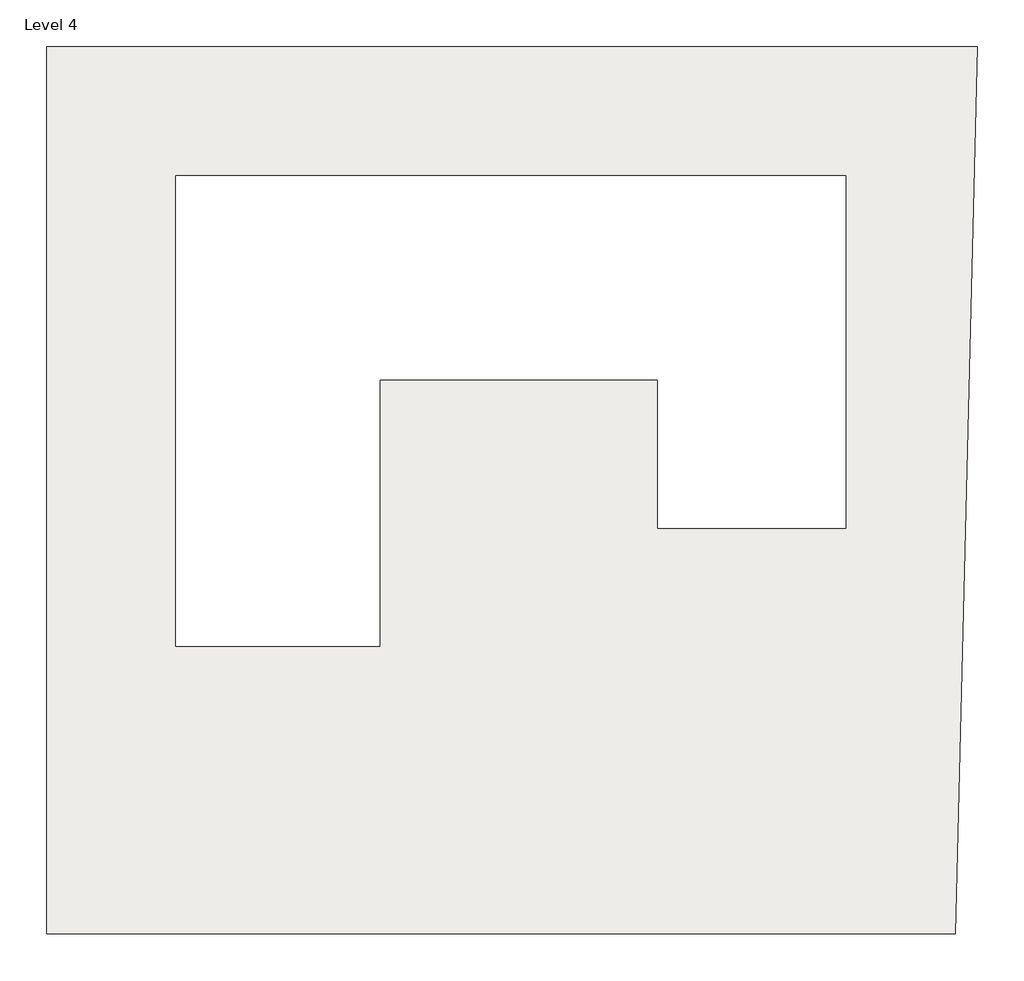
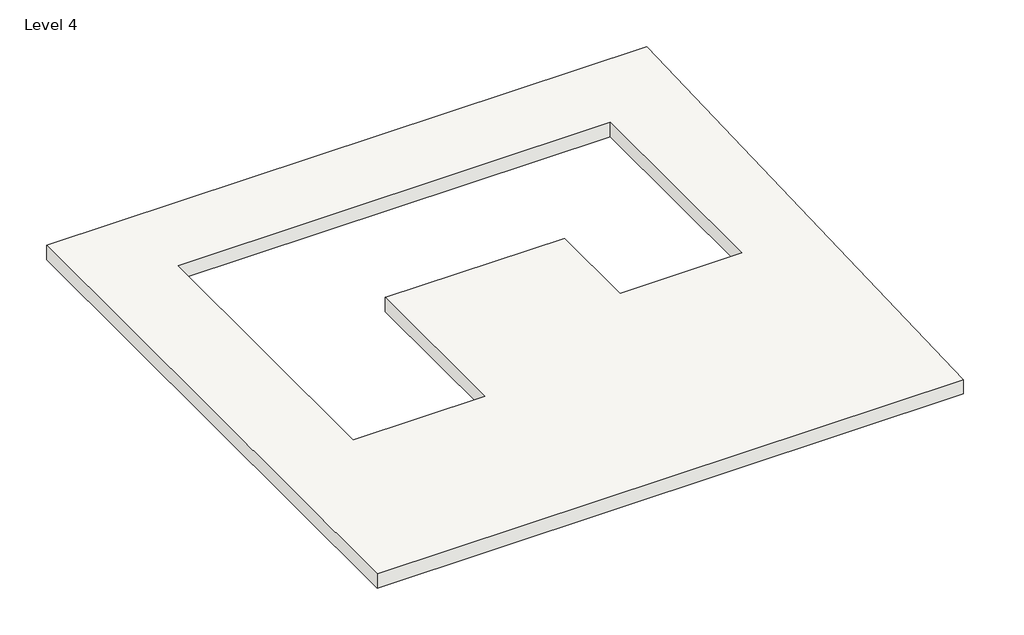
# One storey, incomplete: 1 roof.
"""IFC4 building model written with IfcOpenShell, lengths in millimetres."""

from ifc_helpers import new_model, si_unit, frame, origin, place, context, project, spatial, polyline, outline, extrude, element, save

model = new_model("IFC4")

# Units and contexts
model_context = context("Model", 3, world=origin())
ifc_project = project(units=[si_unit("LENGTHUNIT", "METRE", prefix="MILLI")], contexts=[model_context])

# Site, building, storey
site = spatial("IfcSite", under=ifc_project)
building = spatial("IfcBuilding", under=site)
storey = spatial("IfcBuildingStorey", under=building, Name="Level 4", Elevation=9448.8)

# Roof
placement = place(None, origin())
element("IfcRoof", 1, ObjectType="ROOF 6\"", at=placement, inside=storey, context=model_context, shape_type="SweptSolid", body=[
    extrude(outline(polyline([(-35576.4449318, 16573.1618061), (-35721.4810662, 10820.0618061), (-41611.3146233, 10820.0618061), (-41611.3146233, 16573.1618061), (-35576.4449318, 16573.1618061)]), holes=[polyline([(-39452.3146233, 12686.9618061), (-39452.3146233, 14414.1618061), (-37648.9146233, 14414.1618061), (-37648.9146233, 13448.9618061), (-36429.7146233, 13448.9618061), (-36429.7146233, 15734.9618061), (-40773.1146233, 15734.9618061), (-40773.1146233, 12686.9618061), (-39452.3146233, 12686.9618061)])]), frame((0.0, 0.0, 9296.4), z_axis=(0.0, 0.0, 1.0), x_axis=(1.0, 0.0, 0.0)), (0.0, 0.0, 1.0), 152.4),
])

save(model, "model.ifc")

# Revit data of these elements
# Type "ROOF 6\""
#   Assembly Code = "B1020"
#   Layers, outside or top first: 0' - 6" no material (function 1)
# Element 1 (IfcRoof, "ROOF 6\"")
#   built-in parameter 1001705 = 31 (stored number, unit not read)
#   built-in parameter 1001701 = -0.5 (stored number, unit not read)
#   built-in parameter 1001710 = 33615
#   Phase Created = New Construction
#   Materials on its faces: "Default Roof", "Copper", "Wood - Stained"
# Materials
#   "Default Roof": colour RGB 88 101 114, transparency 0, Cost = 0
#   "Copper": class "Metal", colour RGB 0 0 0, transparency 0, Description = "Copper, matte finish", Cost = 0
#   "Wood - Stained": class "Wood", colour RGB 224 178 126, transparency 0, Cost = 0
